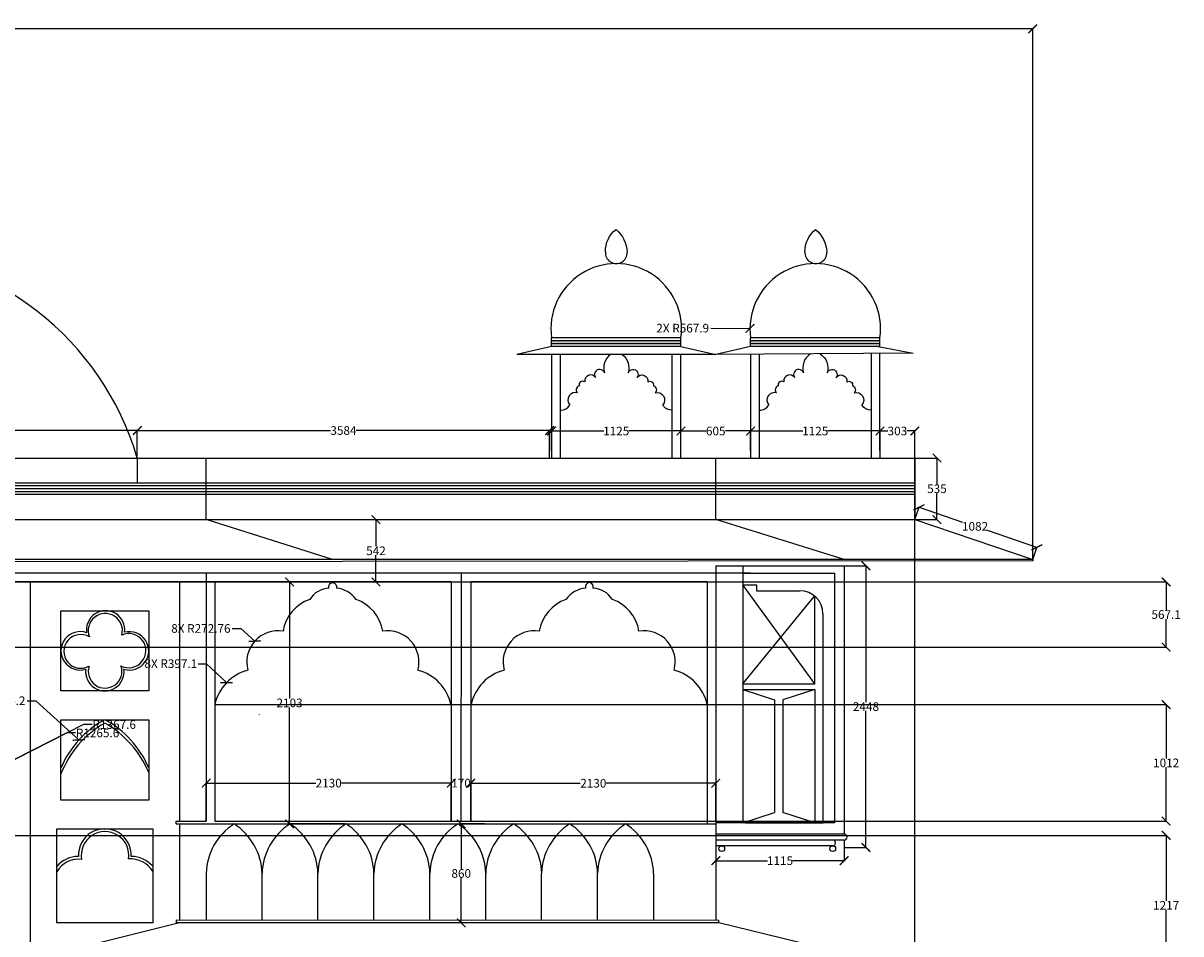
# Model space of a CAD drawing. Units: inches. Extents: x 829 to 33356404, y 1874 to 16983.
# Tile 9 of 9: x 16199 to 26262, y 9069 to 16983. Entities that reach past the tile are written whole.
import ezdxf

# ---------------------------------------------------------------- set-up
doc = ezdxf.new("R2010")
doc.units = ezdxf.units.IN
doc.header["$MEASUREMENT"] = 0
doc.header["$PDMODE"] = 3
for name, color, linetype, lineweight in [('A-ANNO-DIMS', 2, 'Continuous', 18), ('A-ELEV', 7, 'Continuous', 25), ('A-ELEV-PATT', 8, 'Continuous', 13)]:
    doc.layers.add(name, color=color, linetype=linetype, lineweight=lineweight)
doc.styles.get("Standard").update_dxf_attribs({"font": 'arial.ttf'})
doc.dimstyles.get("Standard").update_dxf_attribs({"dimtxt": 75, "dimasz": 75, "dimexe": 0.18, "dimexo": 0.0625, "dimgap": 0.09, "dimtad": 0, "dimtih": 1, "dimtoh": 1, "dimdec": 0, "dimzin": 0, "dimdsep": 46, "dimtxsty": 'Standard', "dimblk": 'ARCHTICK', "dimcen": 0.09, "dimadec": 0, "dimazin": 0, "dimtfac": 1, "dimtdec": 0, "dimtofl": 0, "dimtmove": 0, "dimatfit": 3, "dimfxl": 1, "dimtolj": 1, "dimtzin": 0, "dimarcsym": 0})

# ---------------------------------------------------------------- blocks, each defined once
blk = doc.blocks.new('_ArchTick')
at = {"color": 0, "linetype": 'ByBlock', "const_width": 0.15}
blk.add_lwpolyline([(-0.5, -0.5), (0.5, 0.5)], dxfattribs=at)
blk = doc.blocks.new('*D14')
at = {"layer": 'A-ANNO-DIMS', "color": 0, "lineweight": -2, "transparency": 16777216}
for p, q in [((18994, 12127), (18515, 12127)), ((18515, 12127), (18515, 11114)), ((18515, 10024), (18515, 11037)), ((18994, 10024), (18515, 10024))]:
    blk.add_line(p, q, dxfattribs=at)
at = {"layer": 'Defpoints', "color": 0, "transparency": 16777216}
for p in [(18515, 12127), (18994, 12127), (18994, 10024)]:
    blk.add_point(p, dxfattribs=at)
at = {"layer": 'A-ANNO-DIMS', "color": 0, "lineweight": -2, "transparency": 16777216, "xscale": 75, "yscale": 75, "zscale": 75}
for p, rotation in [((18515, 12127), 90), ((18515, 10024), 270)]:
    blk.add_blockref('_ArchTick', p, dxfattribs=dict(at, rotation=rotation))
at = {"layer": 'A-ANNO-DIMS', "color": 0, "transparency": 16777216, "insert": (18515, 11076), "char_height": 75, "attachment_point": 5}
blk.add_mtext('\\A1;2103', dxfattribs=at)
blk = doc.blocks.new('*D15')
at = {"layer": 'A-ANNO-DIMS', "color": 0, "lineweight": -2, "transparency": 16777216}
for p, q in [((23335, 9884), (23335, 9705)), ((22220, 9819), (22220, 9705)), ((22220, 9705), (22669, 9705)), ((23335, 9705), (22887, 9705))]:
    blk.add_line(p, q, dxfattribs=at)
at = {"layer": 'Defpoints', "color": 0, "transparency": 16777216}
for p in [(23335, 9884), (22220, 9820), (23335, 9705)]:
    blk.add_point(p, dxfattribs=at)
at = {"layer": 'A-ANNO-DIMS', "color": 0, "lineweight": -2, "transparency": 16777216, "xscale": 75, "yscale": 75, "zscale": 75, "rotation": 180}
blk.add_blockref('_ArchTick', (22220, 9705), dxfattribs=at)
at = {"layer": 'A-ANNO-DIMS', "color": 0, "lineweight": -2, "transparency": 16777216, "xscale": 75, "yscale": 75, "zscale": 75}
blk.add_blockref('_ArchTick', (23335, 9705), dxfattribs=at)
at = {"layer": 'A-ANNO-DIMS', "color": 0, "transparency": 16777216, "insert": (22778, 9705), "char_height": 75, "attachment_point": 5}
blk.add_mtext('\\A1;1115', dxfattribs=at)
blk = doc.blocks.new('*D16')
at = {"layer": 'A-ANNO-DIMS', "color": 0, "lineweight": -2, "transparency": 16777216}
for p, q in [((23336, 12268), (23526, 12268)), ((23525, 12268), (23525, 11082)), ((23525, 9820), (23525, 11006)), ((23336, 9820), (23526, 9820))]:
    blk.add_line(p, q, dxfattribs=at)
at = {"layer": 'Defpoints', "color": 0, "transparency": 16777216}
for p in [(23335, 12268), (23525, 12268), (23335, 9820)]:
    blk.add_point(p, dxfattribs=at)
at = {"layer": 'A-ANNO-DIMS', "color": 0, "lineweight": -2, "transparency": 16777216, "xscale": 75, "yscale": 75, "zscale": 75}
for p, rotation in [((23525, 12268), 90), ((23525, 9820), 270)]:
    blk.add_blockref('_ArchTick', p, dxfattribs=dict(at, rotation=rotation))
at = {"layer": 'A-ANNO-DIMS', "color": 0, "transparency": 16777216, "insert": (23525, 11044), "char_height": 75, "attachment_point": 5}
blk.add_mtext('\\A1;2448', dxfattribs=at)
blk = doc.blocks.new('*D25')
at = {"layer": 'A-ANNO-DIMS', "color": 0, "lineweight": -2, "transparency": 16777216}
for p, q in [((20090, 10049), (20090, 10379)), ((20090, 10378), (21042, 10378)), ((22220, 10378), (21268, 10378)), ((22220, 10049), (22220, 10379))]:
    blk.add_line(p, q, dxfattribs=at)
at = {"layer": 'Defpoints', "color": 0, "transparency": 16777216}
for p in [(22220, 10378), (20090, 10049), (22220, 10049)]:
    blk.add_point(p, dxfattribs=at)
at = {"layer": 'A-ANNO-DIMS', "color": 0, "lineweight": -2, "transparency": 16777216, "xscale": 75, "yscale": 75, "zscale": 75, "rotation": 180}
blk.add_blockref('_ArchTick', (20090, 10378), dxfattribs=at)
at = {"layer": 'A-ANNO-DIMS', "color": 0, "lineweight": -2, "transparency": 16777216, "xscale": 75, "yscale": 75, "zscale": 75}
blk.add_blockref('_ArchTick', (22220, 10378), dxfattribs=at)
at = {"layer": 'A-ANNO-DIMS', "color": 0, "transparency": 16777216, "insert": (21155, 10378), "char_height": 75, "attachment_point": 5}
blk.add_mtext('\\A1;2130', dxfattribs=at)
blk = doc.blocks.new('*D26')
at = {"layer": 'A-ANNO-DIMS', "color": 0, "lineweight": -2, "transparency": 16777216}
for p, q in [((17790, 10049), (17790, 10379)), ((17790, 10379), (18742, 10379)), ((19920, 10379), (18967, 10379)), ((19920, 10049), (19920, 10379))]:
    blk.add_line(p, q, dxfattribs=at)
at = {"layer": 'Defpoints', "color": 0, "transparency": 16777216}
for p in [(19920, 10379), (17790, 10049), (19920, 10049)]:
    blk.add_point(p, dxfattribs=at)
at = {"layer": 'A-ANNO-DIMS', "color": 0, "lineweight": -2, "transparency": 16777216, "xscale": 75, "yscale": 75, "zscale": 75, "rotation": 180}
blk.add_blockref('_ArchTick', (17790, 10379), dxfattribs=at)
at = {"layer": 'A-ANNO-DIMS', "color": 0, "lineweight": -2, "transparency": 16777216, "xscale": 75, "yscale": 75, "zscale": 75}
blk.add_blockref('_ArchTick', (19920, 10379), dxfattribs=at)
at = {"layer": 'A-ANNO-DIMS', "color": 0, "transparency": 16777216, "insert": (18855, 10379), "char_height": 75, "attachment_point": 5}
blk.add_mtext('\\A1;2130', dxfattribs=at)
blk = doc.blocks.new('*D27')
at = {"layer": 'A-ANNO-DIMS', "color": 0, "lineweight": -2, "transparency": 16777216}
for p, q in [((19920, 10049), (19920, 10379)), ((19920, 10379), (19926, 10379)), ((20090, 10379), (20084, 10379)), ((20090, 10049), (20090, 10379))]:
    blk.add_line(p, q, dxfattribs=at)
at = {"layer": 'Defpoints', "color": 0, "transparency": 16777216}
for p in [(20090, 10379), (19920, 10049), (20090, 10049)]:
    blk.add_point(p, dxfattribs=at)
at = {"layer": 'A-ANNO-DIMS', "color": 0, "lineweight": -2, "transparency": 16777216, "xscale": 75, "yscale": 75, "zscale": 75, "rotation": 180}
blk.add_blockref('_ArchTick', (19920, 10379), dxfattribs=at)
at = {"layer": 'A-ANNO-DIMS', "color": 0, "lineweight": -2, "transparency": 16777216, "xscale": 75, "yscale": 75, "zscale": 75}
blk.add_blockref('_ArchTick', (20090, 10379), dxfattribs=at)
at = {"layer": 'A-ANNO-DIMS', "color": 0, "transparency": 16777216, "insert": (20005, 10379), "char_height": 75, "attachment_point": 5}
blk.add_mtext('\\A1;170', dxfattribs=at)
blk = doc.blocks.new('*D28')
at = {"layer": 'A-ANNO-DIMS', "color": 0, "lineweight": -2, "transparency": 16777216}
for p, q in [((19162, 12669), (19266, 12669)), ((19266, 12669), (19266, 12437)), ((19266, 12127), (19266, 12360)), ((19162, 12127), (19266, 12127))]:
    blk.add_line(p, q, dxfattribs=at)
at = {"layer": 'Defpoints', "color": 0, "transparency": 16777216}
for p in [(19162, 12669), (19266, 12669), (19162, 12127)]:
    blk.add_point(p, dxfattribs=at)
at = {"layer": 'A-ANNO-DIMS', "color": 0, "lineweight": -2, "transparency": 16777216, "xscale": 75, "yscale": 75, "zscale": 75}
for p, rotation in [((19266, 12669), 90), ((19266, 12127), 270)]:
    blk.add_blockref('_ArchTick', p, dxfattribs=dict(at, rotation=rotation))
at = {"layer": 'A-ANNO-DIMS', "color": 0, "transparency": 16777216, "insert": (19266, 12398), "char_height": 75, "attachment_point": 5}
blk.add_mtext('\\A1;542', dxfattribs=at)
blk = doc.blocks.new('*D50')
at = {"layer": 'A-ANNO-DIMS', "color": 0, "lineweight": -2, "transparency": 16777216}
for p, q in [((22522, 13270), (22522, 13439)), ((22522, 13439), (22975, 13439)), ((23647, 13439), (23193, 13439)), ((23647, 13270), (23647, 13439))]:
    blk.add_line(p, q, dxfattribs=at)
at = {"layer": 'Defpoints', "color": 0, "transparency": 16777216}
for p in [(22522, 13439), (22522, 13269), (23647, 13269)]:
    blk.add_point(p, dxfattribs=at)
at = {"layer": 'A-ANNO-DIMS', "color": 0, "lineweight": -2, "transparency": 16777216, "xscale": 75, "yscale": 75, "zscale": 75, "rotation": 180}
blk.add_blockref('_ArchTick', (22522, 13439), dxfattribs=at)
at = {"layer": 'A-ANNO-DIMS', "color": 0, "lineweight": -2, "transparency": 16777216, "xscale": 75, "yscale": 75, "zscale": 75}
blk.add_blockref('_ArchTick', (23647, 13439), dxfattribs=at)
at = {"layer": 'A-ANNO-DIMS', "color": 0, "transparency": 16777216, "insert": (23084, 13439), "char_height": 75, "attachment_point": 5}
blk.add_mtext('\\A1;1125', dxfattribs=at)
blk = doc.blocks.new('*D49')
at = {"layer": 'A-ANNO-DIMS', "color": 0, "lineweight": -2, "transparency": 16777216}
for p, q in [((21917, 13270), (21917, 13439)), ((21917, 13439), (22136, 13439)), ((22522, 13439), (22303, 13439)), ((22522, 13270), (22522, 13439))]:
    blk.add_line(p, q, dxfattribs=at)
at = {"layer": 'Defpoints', "color": 0, "transparency": 16777216}
for p in [(21917, 13439), (21917, 13269), (22522, 13269)]:
    blk.add_point(p, dxfattribs=at)
at = {"layer": 'A-ANNO-DIMS', "color": 0, "lineweight": -2, "transparency": 16777216, "xscale": 75, "yscale": 75, "zscale": 75, "rotation": 180}
blk.add_blockref('_ArchTick', (21917, 13439), dxfattribs=at)
at = {"layer": 'A-ANNO-DIMS', "color": 0, "lineweight": -2, "transparency": 16777216, "xscale": 75, "yscale": 75, "zscale": 75}
blk.add_blockref('_ArchTick', (22522, 13439), dxfattribs=at)
at = {"layer": 'A-ANNO-DIMS', "color": 0, "transparency": 16777216, "insert": (22219, 13439), "char_height": 75, "attachment_point": 5}
blk.add_mtext('\\A1;605', dxfattribs=at)
blk = doc.blocks.new('*D51')
at = {"layer": 'A-ANNO-DIMS', "color": 0, "lineweight": -2, "transparency": 16777216}
for p, q in [((20792, 13270), (20792, 13439)), ((20792, 13439), (21245, 13439)), ((21917, 13439), (21463, 13439)), ((21917, 13270), (21917, 13439))]:
    blk.add_line(p, q, dxfattribs=at)
at = {"layer": 'Defpoints', "color": 0, "transparency": 16777216}
for p in [(20792, 13439), (20792, 13269), (21917, 13269)]:
    blk.add_point(p, dxfattribs=at)
at = {"layer": 'A-ANNO-DIMS', "color": 0, "lineweight": -2, "transparency": 16777216, "xscale": 75, "yscale": 75, "zscale": 75, "rotation": 180}
blk.add_blockref('_ArchTick', (20792, 13439), dxfattribs=at)
at = {"layer": 'A-ANNO-DIMS', "color": 0, "lineweight": -2, "transparency": 16777216, "xscale": 75, "yscale": 75, "zscale": 75}
blk.add_blockref('_ArchTick', (21917, 13439), dxfattribs=at)
at = {"layer": 'A-ANNO-DIMS', "color": 0, "transparency": 16777216, "insert": (21354, 13439), "char_height": 75, "attachment_point": 5}
blk.add_mtext('\\A1;1125', dxfattribs=at)
blk = doc.blocks.new('*D52')
at = {"layer": 'A-ANNO-DIMS', "color": 0, "lineweight": -2, "transparency": 16777216}
for p, q in [((23950, 12669), (23986, 12776)), ((23986, 12776), (24365, 12647)), ((25010, 12428), (24581, 12574)), ((24974, 12321), (25010, 12428))]:
    blk.add_line(p, q, dxfattribs=at)
at = {"layer": 'Defpoints', "color": 0, "transparency": 16777216}
for p in [(23950, 12669), (25010, 12428), (24974, 12321)]:
    blk.add_point(p, dxfattribs=at)
at = {"layer": 'A-ANNO-DIMS', "color": 0, "lineweight": -2, "transparency": 16777216, "xscale": 75, "yscale": 75, "zscale": 75}
for p, rotation in [((23986, 12776), 161.2250279708252), ((25010, 12428), 341.2250279708252)]:
    blk.add_blockref('_ArchTick', p, dxfattribs=dict(at, rotation=rotation))
at = {"layer": 'A-ANNO-DIMS', "color": 0, "transparency": 16777216, "insert": (24473, 12610), "char_height": 75, "attachment_point": 5}
blk.add_mtext('\\A1;1082', dxfattribs=at)
blk = doc.blocks.new('*D53')
at = {"layer": 'A-ANNO-DIMS', "color": 0, "lineweight": -2, "transparency": 16777216}
for p, q in [((23950, 13204), (24142, 13204)), ((24142, 13204), (24142, 12975)), ((24142, 12669), (24142, 12898)), ((23950, 12669), (24142, 12669))]:
    blk.add_line(p, q, dxfattribs=at)
at = {"layer": 'Defpoints', "color": 0, "transparency": 16777216}
for p in [(23950, 13204), (23950, 12669), (24142, 12669)]:
    blk.add_point(p, dxfattribs=at)
at = {"layer": 'A-ANNO-DIMS', "color": 0, "lineweight": -2, "transparency": 16777216, "xscale": 75, "yscale": 75, "zscale": 75}
for p, rotation in [((24142, 13204), 90), ((24142, 12669), 270)]:
    blk.add_blockref('_ArchTick', p, dxfattribs=dict(at, rotation=rotation))
at = {"layer": 'A-ANNO-DIMS', "color": 0, "transparency": 16777216, "insert": (24142, 12937), "char_height": 75, "attachment_point": 5}
blk.add_mtext('\\A1;535', dxfattribs=at)
blk = doc.blocks.new('*D55')
at = {"layer": 'A-ANNO-DIMS', "color": 0, "lineweight": -2, "transparency": 16777216}
for p, q in [((9931, 13204), (9931, 13443)), ((9931, 13443), (13449, 13443)), ((17191, 13443), (13672, 13443)), ((17191, 13204), (17191, 13443))]:
    blk.add_line(p, q, dxfattribs=at)
at = {"layer": 'Defpoints', "color": 0, "transparency": 16777216}
for p in [(17191, 13443), (9931, 13204), (17191, 13204)]:
    blk.add_point(p, dxfattribs=at)
at = {"layer": 'A-ANNO-DIMS', "color": 0, "lineweight": -2, "transparency": 16777216, "xscale": 75, "yscale": 75, "zscale": 75, "rotation": 180}
blk.add_blockref('_ArchTick', (9931, 13443), dxfattribs=at)
at = {"layer": 'A-ANNO-DIMS', "color": 0, "lineweight": -2, "transparency": 16777216, "xscale": 75, "yscale": 75, "zscale": 75}
blk.add_blockref('_ArchTick', (17191, 13443), dxfattribs=at)
at = {"layer": 'A-ANNO-DIMS', "color": 0, "transparency": 16777216, "insert": (13561, 13443), "char_height": 75, "attachment_point": 5}
blk.add_mtext('\\A1;7260', dxfattribs=at)
blk = doc.blocks.new('*D58')
at = {"layer": 'A-ANNO-DIMS', "color": 0, "lineweight": -2, "transparency": 16777216}
for p, q in [((23647, 13204), (23647, 13439)), ((23647, 13439), (23715, 13439)), ((23950, 13439), (23881, 13439)), ((23950, 13204), (23950, 13439))]:
    blk.add_line(p, q, dxfattribs=at)
at = {"layer": 'Defpoints', "color": 0, "transparency": 16777216}
for p in [(23647, 13439), (23647, 13204), (23950, 13204)]:
    blk.add_point(p, dxfattribs=at)
at = {"layer": 'A-ANNO-DIMS', "color": 0, "lineweight": -2, "transparency": 16777216, "xscale": 75, "yscale": 75, "zscale": 75, "rotation": 180}
blk.add_blockref('_ArchTick', (23647, 13439), dxfattribs=at)
at = {"layer": 'A-ANNO-DIMS', "color": 0, "lineweight": -2, "transparency": 16777216, "xscale": 75, "yscale": 75, "zscale": 75}
blk.add_blockref('_ArchTick', (23950, 13439), dxfattribs=at)
at = {"layer": 'A-ANNO-DIMS', "color": 0, "transparency": 16777216, "insert": (23798, 13439), "char_height": 75, "attachment_point": 5}
blk.add_mtext('\\A1;303', dxfattribs=at)
blk = doc.blocks.new('*D65')
at = {"layer": 'A-ANNO-DIMS', "color": 0, "lineweight": -2, "transparency": 16777216}
for p, q in [((20209, 10024), (20007, 10024)), ((20007, 10024), (20007, 9632)), ((20007, 9164), (20007, 9556)), ((20209, 9164), (20007, 9164))]:
    blk.add_line(p, q, dxfattribs=at)
at = {"layer": 'Defpoints', "color": 0, "transparency": 16777216}
for p in [(20209, 10024), (20007, 9164), (20209, 9164)]:
    blk.add_point(p, dxfattribs=at)
at = {"layer": 'A-ANNO-DIMS', "color": 0, "lineweight": -2, "transparency": 16777216, "xscale": 75, "yscale": 75, "zscale": 75}
for p, rotation in [((20007, 10024), 90), ((20007, 9164), 270)]:
    blk.add_blockref('_ArchTick', p, dxfattribs=dict(at, rotation=rotation))
at = {"layer": 'A-ANNO-DIMS', "color": 0, "transparency": 16777216, "insert": (20007, 9594), "char_height": 75, "attachment_point": 5}
blk.add_mtext('\\A1;860', dxfattribs=at)
blk = doc.blocks.new('*D66')
at = {"layer": 'A-ANNO-DIMS', "color": 0, "lineweight": -2, "transparency": 16777216}
for p, q in [((17191, 13204), (17191, 13443)), ((17191, 13443), (18871, 13443)), ((20775, 13443), (19095, 13443)), ((20775, 13204), (20775, 13443))]:
    blk.add_line(p, q, dxfattribs=at)
at = {"layer": 'Defpoints', "color": 0, "transparency": 16777216}
for p in [(20775, 13443), (17191, 13204), (20775, 13204)]:
    blk.add_point(p, dxfattribs=at)
at = {"layer": 'A-ANNO-DIMS', "color": 0, "lineweight": -2, "transparency": 16777216, "xscale": 75, "yscale": 75, "zscale": 75, "rotation": 180}
blk.add_blockref('_ArchTick', (17191, 13443), dxfattribs=at)
at = {"layer": 'A-ANNO-DIMS', "color": 0, "lineweight": -2, "transparency": 16777216, "xscale": 75, "yscale": 75, "zscale": 75}
blk.add_blockref('_ArchTick', (20775, 13443), dxfattribs=at)
at = {"layer": 'A-ANNO-DIMS', "color": 0, "transparency": 16777216, "insert": (18983, 13443), "char_height": 75, "attachment_point": 5}
blk.add_mtext('\\A1;3584', dxfattribs=at)
blk = doc.blocks.new('ARCADE-ARCHES')
for p, q in [((0, 405), (0, 0)), ((486, 0), (486, 405)), ((972, 0), (972, 405)), ((1458, 0), (1458, 405)), ((1944, 0), (1944, 405)), ((2430, 0), (2430, 405)), ((2916, 0), (2916, 405)), ((3402, 0), (3402, 405)), ((3889, 405), (3889, 0))]:
    blk.add_line(p, q)
for centre, start, end in [((526, 392), 122.5147, 178.5225), ((-40, 392), 1.4775, 57.4853), ((1012, 392), 122.5147, 178.5225), ((446, 392), 1.4775, 57.4853), ((1498, 392), 122.5147, 178.5225), ((933, 392), 1.4775, 57.4853), ((1984, 392), 122.5147, 178.5225), ((1419, 392), 1.4775, 57.4853), ((2470, 392), 122.5147, 178.5225), ((1905, 392), 1.4775, 57.4853), ((2956, 392), 122.5147, 178.5225), ((2391, 392), 1.4775, 57.4853), ((3442, 392), 122.5147, 178.5225), ((2877, 392), 1.4775, 57.4853), ((3928, 392), 122.5147, 178.5225), ((3363, 392), 1.4775, 57.4853)]:
    blk.add_arc(centre, 526, start, end)
blk = doc.blocks.new('CHHATRI-ARCH-A')
blk.add_lwpolyline([(0, 0, 0.306755), (82, 44, 10.100933)], format="xyb")
for centre, radius, start, end in [((525, 365), 147, 122.4143, 196.9076), ((264, 253), 51.8, 32.9883, 190.2779), ((342, 309), 44.1, 17.6268, 218.3613), ((175, 175), 36.4, 106.3078, 227.8776), ((195, 218), 31.7, 54.8887, 193.7899), ((131, 87), 64.5, 72.3169, 221.8651)]:
    blk.add_arc(centre, radius, start, end)
blk = doc.blocks.new('CHHATRI-ARCH-B')
blk.add_lwpolyline([(0, 0, 0.306755), (82, 44, 10.100933)], format="xyb")
for centre, radius, start, end in [((525, 365), 147, 126.8528, 196.9076), ((264, 253), 51.8, 32.9883, 190.2779), ((342, 309), 44.1, 17.6268, 218.3613), ((175, 175), 36.4, 106.3078, 227.8776), ((195, 218), 31.7, 54.8887, 193.7899), ((131, 87), 64.5, 72.3169, 221.8651)]:
    blk.add_arc(centre, radius, start, end)
blk = doc.blocks.new('*D82')
at = {"layer": 'A-ANNO-DIMS', "color": 0, "lineweight": -2, "transparency": 16777216}
for p, q in [((2146, 12292), (2146, 16934)), ((2146, 16934), (13418, 16934)), ((24974, 16934), (13702, 16934)), ((24974, 12321), (24974, 16934))]:
    blk.add_line(p, q, dxfattribs=at)
at = {"layer": 'Defpoints', "color": 0, "transparency": 16777216}
for p in [(24974, 16934), (2146, 12292), (24974, 12321)]:
    blk.add_point(p, dxfattribs=at)
at = {"layer": 'A-ANNO-DIMS', "color": 0, "lineweight": -2, "transparency": 16777216, "xscale": 75, "yscale": 75, "zscale": 75, "rotation": 180}
blk.add_blockref('_ArchTick', (2146, 16934), dxfattribs=at)
at = {"layer": 'A-ANNO-DIMS', "color": 0, "lineweight": -2, "transparency": 16777216, "xscale": 75, "yscale": 75, "zscale": 75}
blk.add_blockref('_ArchTick', (24974, 16934), dxfattribs=at)
at = {"layer": 'A-ANNO-DIMS', "color": 0, "transparency": 16777216, "insert": (13560, 16934), "char_height": 75, "attachment_point": 5}
blk.add_mtext('\\A1;22828', dxfattribs=at)
blk = doc.blocks.new('*D90')
at = {"layer": 'A-ANNO-DIMS', "color": 0, "lineweight": -2, "transparency": 16777216}
for p, q in [((17865, 11061), (26134, 11061)), ((26134, 11061), (26134, 10594)), ((26134, 10049), (26134, 10517)), ((17865, 10049), (26134, 10049))]:
    blk.add_line(p, q, dxfattribs=at)
at = {"layer": 'Defpoints', "color": 0, "transparency": 16777216}
for p in [(17865, 11061), (26134, 11061), (17865, 10049)]:
    blk.add_point(p, dxfattribs=at)
at = {"layer": 'A-ANNO-DIMS', "color": 0, "lineweight": -2, "transparency": 16777216, "xscale": 75, "yscale": 75, "zscale": 75}
for p, rotation in [((26134, 11061), 90), ((26134, 10049), 270)]:
    blk.add_blockref('_ArchTick', p, dxfattribs=dict(at, rotation=rotation))
at = {"layer": 'A-ANNO-DIMS', "color": 0, "transparency": 16777216, "insert": (26134, 10555), "char_height": 75, "attachment_point": 5}
blk.add_mtext('\\A1;1012', dxfattribs=at)
blk = doc.blocks.new('*D91')
at = {"layer": 'A-ANNO-DIMS', "color": 0, "lineweight": -2, "transparency": 16777216}
for p, q in [((11082, 9925), (26134, 9925)), ((26134, 9925), (26134, 9355)), ((26134, 8708), (26134, 9279)), ((11082, 8708), (26134, 8708))]:
    blk.add_line(p, q, dxfattribs=at)
at = {"layer": 'Defpoints', "color": 0, "transparency": 16777216}
for p in [(11082, 9925), (11082, 8708), (26134, 8708)]:
    blk.add_point(p, dxfattribs=at)
at = {"layer": 'A-ANNO-DIMS', "color": 0, "lineweight": -2, "transparency": 16777216, "xscale": 75, "yscale": 75, "zscale": 75}
for p, rotation in [((26134, 9925), 90), ((26134, 8708), 270)]:
    blk.add_blockref('_ArchTick', p, dxfattribs=dict(at, rotation=rotation))
at = {"layer": 'A-ANNO-DIMS', "color": 0, "transparency": 16777216, "insert": (26134, 9317), "char_height": 75, "attachment_point": 5}
blk.add_mtext('\\A1;1217', dxfattribs=at)
blk = doc.blocks.new('*D93')
at = {"layer": 'A-ANNO-DIMS', "color": 0, "lineweight": -2, "transparency": 16777216}
for p, q in [((10980, 12127), (26134, 12127)), ((26134, 12127), (26134, 11882)), ((26134, 11560), (26134, 11805)), ((11677, 11560), (26134, 11560))]:
    blk.add_line(p, q, dxfattribs=at)
at = {"layer": 'Defpoints', "color": 0, "transparency": 16777216}
for p in [(10980, 12127), (11677, 11560), (26134, 11560)]:
    blk.add_point(p, dxfattribs=at)
at = {"layer": 'A-ANNO-DIMS', "color": 0, "lineweight": -2, "transparency": 16777216, "xscale": 75, "yscale": 75, "zscale": 75}
for p, rotation in [((26134, 12127), 90), ((26134, 11560), 270)]:
    blk.add_blockref('_ArchTick', p, dxfattribs=dict(at, rotation=rotation))
at = {"layer": 'A-ANNO-DIMS', "color": 0, "transparency": 16777216, "insert": (26134, 11844), "char_height": 75, "attachment_point": 5}
blk.add_mtext('\\A1;567.1', dxfattribs=at)
blk = doc.blocks.new('*D110')
at = {"layer": 'A-ANNO-DIMS', "color": 0, "lineweight": -2, "transparency": 16777216}
for p, q in [((17719, 11417), (17794, 11417)), ((17794, 11417), (17966, 11252)), ((18253, 10977), (18253, 10977)), ((18253, 10976), (18253, 10977))]:
    blk.add_line(p, q, dxfattribs=at)
at = {"layer": 'Defpoints', "color": 0, "transparency": 16777216}
for p in [(17966, 11252), (18253, 10977)]:
    blk.add_point(p, dxfattribs=at)
at = {"layer": 'A-ANNO-DIMS', "color": 0, "lineweight": -2, "transparency": 16777216, "xscale": 75, "yscale": 75, "zscale": 75, "rotation": 316.167768460209}
blk.add_blockref('_ArchTick', (17966, 11252), dxfattribs=at)
at = {"layer": 'A-ANNO-DIMS', "color": 0, "transparency": 16777216, "insert": (17483, 11417), "char_height": 75, "attachment_point": 5}
blk.add_mtext('\\A1;8X R397.1', dxfattribs=at)
blk = doc.blocks.new('*D112')
at = {"layer": 'A-ANNO-DIMS', "color": 0, "lineweight": -2, "transparency": 16777216}
for p, q in [((18017, 11723), (18092, 11723)), ((18092, 11723), (18213, 11613)), ((18416, 11431), (18416, 11431)), ((18416, 11431), (18416, 11431))]:
    blk.add_line(p, q, dxfattribs=at)
at = {"layer": 'Defpoints', "color": 0, "transparency": 16777216}
for p in [(18213, 11613), (18416, 11431)]:
    blk.add_point(p, dxfattribs=at)
at = {"layer": 'A-ANNO-DIMS', "color": 0, "lineweight": -2, "transparency": 16777216, "xscale": 75, "yscale": 75, "zscale": 75, "rotation": 317.9756692368}
blk.add_blockref('_ArchTick', (18213, 11613), dxfattribs=at)
at = {"layer": 'A-ANNO-DIMS', "color": 0, "transparency": 16777216, "insert": (17744, 11723), "char_height": 75, "attachment_point": 5}
blk.add_mtext('\\A1;8X R272.76', dxfattribs=at)
blk = doc.blocks.new('*D115')
at = {"layer": 'A-ANNO-DIMS', "color": 0, "lineweight": -2, "transparency": 16777216}
for p, q in [((22176, 14333), (22516, 14330)), ((23084, 14326), (23084, 14326)), ((23084, 14326), (23084, 14326))]:
    blk.add_line(p, q, dxfattribs=at)
at = {"layer": 'Defpoints', "color": 0, "transparency": 16777216}
for p in [(22516, 14330), (23084, 14326)]:
    blk.add_point(p, dxfattribs=at)
at = {"layer": 'A-ANNO-DIMS', "color": 0, "lineweight": -2, "transparency": 16777216, "xscale": 75, "yscale": 75, "zscale": 75, "rotation": 359.558569188689}
blk.add_blockref('_ArchTick', (22516, 14330), dxfattribs=at)
at = {"layer": 'A-ANNO-DIMS', "color": 0, "transparency": 16777216, "insert": (21932, 14333), "char_height": 75, "attachment_point": 5}
blk.add_mtext('\\A1;2X R567.9', dxfattribs=at)
blk = doc.blocks.new('*D125')
at = {"layer": 'A-ANNO-DIMS', "color": 0, "lineweight": -2, "transparency": 16777216}
for p, q in [((16725, 10888), (15993, 10518)), ((16800, 10888), (16725, 10888)), ((14772, 9900), (14773, 9900)), ((14772, 9900), (14772, 9900))]:
    blk.add_line(p, q, dxfattribs=at)
at = {"layer": 'Defpoints', "color": 0, "transparency": 16777216}
for p in [(15993, 10518), (14772, 9900)]:
    blk.add_point(p, dxfattribs=at)
at = {"layer": 'A-ANNO-DIMS', "color": 0, "lineweight": -2, "transparency": 16777216, "xscale": 75, "yscale": 75, "zscale": 75, "rotation": 206.8466405163161}
blk.add_blockref('_ArchTick', (15993, 10518), dxfattribs=at)
at = {"layer": 'A-ANNO-DIMS', "color": 0, "transparency": 16777216, "insert": (16991, 10888), "char_height": 75, "attachment_point": 5}
blk.add_mtext('\\A1;R1367.6', dxfattribs=at)
blk = doc.blocks.new('*D126')
at = {"layer": 'A-ANNO-DIMS', "color": 0, "lineweight": -2, "transparency": 16777216}
for p, q in [((16579, 10815), (15902, 10472)), ((16654, 10815), (16579, 10815)), ((14772, 9900), (14773, 9900)), ((14772, 9900), (14772, 9900))]:
    blk.add_line(p, q, dxfattribs=at)
at = {"layer": 'Defpoints', "color": 0, "transparency": 16777216}
for p in [(15902, 10472), (14772, 9900)]:
    blk.add_point(p, dxfattribs=at)
at = {"layer": 'A-ANNO-DIMS', "color": 0, "lineweight": -2, "transparency": 16777216, "xscale": 75, "yscale": 75, "zscale": 75, "rotation": 206.8466187545911}
blk.add_blockref('_ArchTick', (15902, 10472), dxfattribs=at)
at = {"layer": 'A-ANNO-DIMS', "color": 0, "transparency": 16777216, "insert": (16846, 10815), "char_height": 75, "attachment_point": 5}
blk.add_mtext('\\A1;R1265.6', dxfattribs=at)
blk = doc.blocks.new('*D130')
at = {"layer": 'A-ANNO-DIMS', "color": 0, "lineweight": -2, "transparency": 16777216}
for p, q in [((16233, 11095), (16308, 11095)), ((16308, 11095), (16683, 10754)), ((17306, 10185), (17306, 10185)), ((17306, 10185), (17306, 10185))]:
    blk.add_line(p, q, dxfattribs=at)
at = {"layer": 'Defpoints', "color": 0, "transparency": 16777216}
for p in [(16683, 10754), (17306, 10185)]:
    blk.add_point(p, dxfattribs=at)
at = {"layer": 'A-ANNO-DIMS', "color": 0, "lineweight": -2, "transparency": 16777216, "xscale": 75, "yscale": 75, "zscale": 75, "rotation": 317.6357309782866}
blk.add_blockref('_ArchTick', (16683, 10754), dxfattribs=at)
at = {"layer": 'A-ANNO-DIMS', "color": 0, "transparency": 16777216, "insert": (15989, 11095), "char_height": 75, "attachment_point": 5}
blk.add_mtext('\\A1;4X R844.2', dxfattribs=at)

msp = doc.modelspace()

# ---------------------------------------------------------------- hatches: boundary and pattern name
at = {"layer": 'A-ELEV-PATT'}
h = msp.add_hatch(color=256, dxfattribs=at)
h.dxf.hatch_style = 1
h.paths.add_polyline_path([(20791.778, 14222.485), (21354.278, 14222.485), (21354.278, 14197.485), (20791.778, 14197.485)])
h = msp.add_hatch(color=256, dxfattribs=at)
h.dxf.hatch_style = 1
h.paths.add_polyline_path([(21354.278, 14222.485), (21916.778, 14222.485), (21916.778, 14197.485), (21354.278, 14197.485)])
h = msp.add_hatch(color=256, dxfattribs=at)
h.dxf.hatch_style = 1
h.paths.add_polyline_path([(22521.778, 14222.485), (23084.278, 14222.485), (23084.278, 14197.485), (22521.778, 14197.485)])
h = msp.add_hatch(color=256, dxfattribs=at)
h.dxf.hatch_style = 1
h.paths.add_polyline_path([(23084.278, 14222.485), (23646.778, 14222.485), (23646.778, 14197.485), (23084.278, 14197.485)])

# ---------------------------------------------------------------- linework, layer by layer
at = {"layer": 'A-ELEV'}
for p, q in [((21916.778, 14247.485), (20791.778, 14247.485)), ((20791.778, 14172.485), (20791.778, 14247.485)), ((21916.778, 14222.485), (20791.778, 14222.485)), ((21916.778, 14197.485), (20791.778, 14197.485)), ((21916.778, 14172.485), (21916.778, 14247.485)), ((23646.778, 14247.485), (22521.778, 14247.485)), ((22521.778, 14172.485), (22521.778, 14247.485)), ((23646.778, 14222.485), (22521.778, 14222.485)), ((23646.778, 14197.485), (22521.778, 14197.485)), ((23646.778, 14172.485), (23646.778, 14247.485)), ((20791.778, 14172.485), (20489.778, 14103.629)), ((22219.778, 14103.629), (20489.778, 14103.629)), ((21916.778, 14172.485), (20791.778, 14172.485)), ((20791.778, 14103.629), (20791.778, 13204.032)), ((20866.778, 14103.629), (20866.778, 13204.032)), ((21841.778, 13204.032), (21841.778, 14103.629)), ((21916.778, 14172.485), (22219.778, 14103.629)), ((21916.778, 13204.032), (21916.778, 14103.629)), ((23934.855, 14115.977), (22204.855, 14103.629)), ((22521.778, 14172.485), (22219.778, 14103.629)), ((23646.778, 14172.485), (22521.778, 14172.485)), ((22521.778, 14105.785), (22521.778, 13204.032)), ((22596.778, 14106.32), (22596.778, 13204.032)), ((23571.778, 13204.032), (23571.778, 14113.279)), ((23631.855, 14172.485), (23934.855, 14115.977)), ((23646.778, 13269.485), (23646.778, 14113.814)), ((3169.778, 13204.032), (23949.778, 13204.032)), ((17190.778, 13204.032), (17190.778, 12986.532)), ((17789.778, 12669.032), (17789.778, 13204.032)), ((22219.278, 12669.032), (22219.278, 13204.032)), ((23949.778, 4746.468), (23949.778, 13204.032)), ((23949.778, 13204.032), (23949.778, 12669.032)), ((23949.778, 12986.532), (3169.778, 12986.532)), ((23949.778, 12961.532), (3169.778, 12961.532)), ((23949.778, 12936.532), (3169.778, 12936.532)), ((23949.778, 12911.532), (3169.778, 12911.532)), ((23949.778, 12886.532), (3169.778, 12886.532)), ((3169.778, 12669.032), (23949.778, 12669.032)), ((18889.175, 12320.882), (17789.778, 12669.032)), ((23334.312, 12320.882), (22219.278, 12669.032)), ((23949.778, 12669.032), (24973.928, 12320.882)), ((24973.929, 12320.882), (2145.628, 12320.882)), ((24973.929, 12310.744), (2145.651, 12292.214)), ((24973.929, 12320.882), (24973.929, 12310.744)), ((22522.278, 12202.212), (3169.778, 12202.212)), ((17789.778, 12202.212), (17789.778, 10049.392)), ((20005.152, 12202.212), (20004.887, 10049.392)), ((22220.173, 12267.948), (22220.173, 9188.877)), ((22220.173, 12267.948), (23335.46, 12267.948)), ((22453.965, 12267.948), (22453.965, 10034.257)), ((22453.965, 12202.212), (23250.93, 12202.212)), ((23250.93, 12202.212), (23250.93, 10034.257)), ((23335.46, 12267.948), (23335.46, 9934.257)), ((18091.883, 12127.212), (9559.826, 12127.212)), ((16258.701, 12127.212), (16258.701, 5024.468)), ((17559.778, 10049.392), (17559.778, 12127.212)), ((17864.778, 12127.212), (17864.778, 10049.392)), ((19919.89, 12127.212), (17864.778, 12127.212)), ((19919.89, 12127.212), (19919.89, 10049.392)), ((20089.89, 12127.212), (20089.89, 10049.392)), ((22144.778, 12127.212), (20089.89, 12127.212)), ((22144.778, 12127.212), (22144.778, 10023.842)), ((22453.965, 12100.687), (22453.965, 12100.687)), ((22453.965, 12100.687), (22574.779, 12100.687)), ((23079.354, 11242.683), (22453.965, 12100.687)), ((22574.779, 12100.687), (22574.779, 12049.925)), ((22453.965, 11242.683), (23077.598, 12004.701)), ((22574.779, 12049.925), (22574.779, 12049.925)), ((22574.779, 12049.925), (22950.93, 12049.925)), ((23079.331, 11242.683), (23079.331, 12004.367)), ((23150.93, 11849.925), (23150.93, 11754.206)), ((23150.93, 11806.442), (23150.93, 10034.257)), ((22453.965, 11242.683), (23079.354, 11242.683)), ((22453.965, 11242.683), (22453.965, 11242.683)), ((22453.965, 11191.921), (23079.354, 11191.921)), ((22453.965, 11191.921), (22731.126, 11101.847)), ((23079.354, 11191.921), (22802.193, 11101.847)), ((23079.354, 11191.921), (23079.354, 10034.257)), ((22731.126, 11101.847), (22731.126, 10124.33)), ((22802.193, 11101.847), (22802.193, 10124.33)), ((22453.965, 10034.257), (22731.126, 10124.33)), ((23079.354, 10034.257), (22802.193, 10124.33)), ((17530.231, 10049.392), (17789.778, 10049.392)), ((17530.231, 10024.454), (17530.231, 10049.392)), ((17530.231, 10024.454), (22220.173, 10023.833)), ((17559.778, 9189.453), (17559.778, 10024.45)), ((17864.778, 10049.392), (22144.89, 10049.392)), ((23250.93, 10034.257), (22220.46, 10034.257)), ((22476.056, 10034.257), (23152.207, 10034.257)), ((23335.46, 9934.257), (22220.46, 9934.257)), ((23335.46, 9884.257), (22220.46, 9884.257)), ((23235.46, 9834.257), (22220.46, 9834.257)), ((17559.22, 9165.468), (16492.651, 8897.385)), ((17530.231, 9189.457), (22247.133, 9188.874)), ((17530.231, 9189.457), (17530.231, 9165.468)), ((22247.13, 9165.468), (17530.231, 9165.468)), ((22247.13, 9165.468), (22247.133, 9188.874)), ((23335.316, 8897.468), (22247.13, 9165.468))]:
    msp.add_line(p, q, dxfattribs=at)
for points in [[(21259.732, 14996.8, -0.235502326), (21352.151, 15190.287, -0.2104826), (21449.057, 14993.527, -0.234209501)], [(22994.733, 14996.669, -0.235502326), (23087.152, 15190.156, -0.2104826), (23184.058, 14993.397, -0.234209501)], [(21349.279, 14893.654, -0.000002916), (21349.277, 14893.653, -0.000003298), (21349.275, 14893.655)], [(23084.28, 14893.524, -0.000002916), (23084.278, 14893.523, -0.000003298), (23084.276, 14893.524)], [(18856.859, 12073.468, -0.442920108), (18891.241, 12123.624, -0.367737881), (18923.182, 12073.468, -0.247488348)], [(21153.177, 12073.468, 0.442920108), (21118.795, 12123.624, 0.367737881), (21086.854, 12073.468, 0.247488348)]]:
    msp.add_lwpolyline(points, format="xyb", dxfattribs=at)
for points in [[(16528.074, 11877.212), (17290.405, 11877.212), (17290.405, 11179.704), (16528.074, 11179.704)], [(16528.074, 10929.704), (17290.405, 10929.704), (17290.405, 10232.196), (16528.074, 10232.196)], [(16492.651, 9982.196), (17325.828, 9982.196), (17325.828, 9165.468), (16492.651, 9165.468)]]:
    msp.add_lwpolyline(points, close=True, dxfattribs=at)
for centre in [(22271.167, 9809.257), (23235.552, 9809.257)]:
    msp.add_circle(centre, 25, dxfattribs=at)
for centre, radius, start, end in [((14785.821, 12499.606), 2506, 16.3256048, 87.9689122), ((21354.278, 14988.438), 94.915, 174.9458751, 3.0734321), ((23089.279, 14988.308), 94.915, 174.9458751, 3.0734321), ((21354.278, 14325.622), 567.901, 352.0917127, 187.9082873), ((23084.278, 14325.622), 567.901, 352.0917127, 187.9082873), ((18807.214, 11640.647), 354.179, 109.4034394, 170.3116953), ((18866.872, 11865.187), 208.419, 92.0817943, 148.2984828), ((18901.683, 11841.246), 233.215, 34.9091215, 84.7106013), ((18975.269, 11640.647), 354.179, 9.6883047, 70.5965606), ((21034.767, 11640.647), 354.179, 109.4034394, 170.3116953), ((21108.353, 11841.246), 233.215, 95.2893987, 145.0908785), ((21143.164, 11865.187), 208.419, 31.7015172, 87.9182057), ((21202.822, 11640.647), 354.179, 9.6883047, 70.5965606), ((22950.93, 11849.925), 200, 0, 90), ((16915.996, 11710.622), 166.726, 352.8036552, 188.7161935), ((16913.34, 11704.536), 148.406, 344.8754049, 201.7505434), ((16694.801, 11528.458), 166.726, 70.2299001, 287.1891398), ((17117.42, 11530.089), 148.727, 242.8881159, 114.1355922), ((17123.679, 11528.458), 166.726, 252.8108602, 104.6864663), ((18415.703, 11430.806), 272.758, 81.0607154, 194.8907352), ((19366.78, 11430.806), 272.758, 345.1092648, 98.9392846), ((20643.256, 11430.806), 272.758, 81.0607154, 194.8907352), ((21594.333, 11430.806), 272.758, 345.1092648, 98.9392846), ((16699.57, 11523.821), 146.871, 58.8698998, 299.852673), ((16911.373, 11350.379), 146.143, 161.6289467, 18.8945071), ((16909.24, 11346.43), 166.726, 172.1579984, 7.8420016), ((18252.722, 10976.551), 397.12, 104.6768994, 167.65861), ((19529.761, 10976.551), 397.12, 12.34139, 75.3231006), ((20480.275, 10976.551), 397.12, 104.6768994, 167.65861), ((21757.314, 10976.551), 397.12, 12.34139, 75.3231006), ((17306.384, 10184.731), 844.22, 118.0620346, 157.2094631), ((17332.151, 10151.495), 860.805, 119.4258677, 159.0828764), ((16512.095, 10184.731), 844.22, 22.7905369, 61.9379654), ((16457.563, 10115.752), 906.1, 23.1978992, 60.1002346), ((16909.24, 9752.067), 230.168, 357.3160887, 182.6839113), ((16910.573, 9749.866), 207.419, 351.6467456, 189.2312463), ((23235.46, 9859.257), 25, 270, 90), ((23335.46, 9909.257), 25, 270, 90), ((16675.101, 9508.068), 233.259, 88.9625622, 141.4604412), ((16678.821, 9506.158), 212.161, 82.6833719, 151.3414814), ((17132.45, 9492.24), 228.102, 32.0298486, 94.1878817), ((17140.006, 9496.16), 245.131, 40.7070038, 90.1988869)]:
    msp.add_arc(centre, radius, start, end, dxfattribs=at)

# ---------------------------------------------------------------- block references
for name, p in [('CHHATRI-ARCH-B', (20867.778, 13621.512)), ('ARCADE-ARCHES', (17789.673, 9188.901))]:
    msp.add_blockref(name, p, dxfattribs=at)
at = {"layer": 'A-ELEV', "extrusion": (0, 0, -1), "zscale": -1}
for name, p in [('CHHATRI-ARCH-B', (-21841.778, 13621.512)), ('CHHATRI-ARCH-A', (-23571.778, 13621.513))]:
    msp.add_blockref(name, p, dxfattribs=at)
at = {"layer": 'A-ELEV', "rotation": 0.0409553348768901}
msp.add_blockref('CHHATRI-ARCH-A', (22597.845, 13621.386), dxfattribs=at)

# ---------------------------------------------------------------- dimensions: what is measured, and where the dimension line sits
at = {"layer": 'A-ANNO-DIMS'}
for base, p1, p2, override, picture, middle in [((24973.929, 16934.032), (2145.651, 12292.214), (24973.929, 12320.882), {"dimdec": 0, "dimlfac": 1, "dimrnd": 0, "dimzin": 0, "dimdsep": 46, "dimlunit": 2}, '*D82', (13559.79, 16934.032)), ((17190.778, 13442.842), (9930.778, 13204.032), (17190.778, 13204.032), {"dimclrd": 0, "dimclre": 0, "dimclrt": 0}, '*D55', (13560.778, 13442.842)), ((20774.778, 13442.842), (17190.778, 13204.032), (20774.778, 13204.032), {"dimclrd": 0, "dimclre": 0, "dimclrt": 0}, '*D66', (18982.778, 13442.842)), ((23646.778, 13438.732), (23949.778, 13204.032), (23646.778, 13204.032), {"dimclrd": 0, "dimclre": 0, "dimclrt": 0}, '*D58', (23798.278, 13438.732)), ((19919.89, 10378.856), (17789.778, 10049.392), (19919.89, 10049.392), {"dimclrd": 0, "dimclre": 0, "dimclrt": 0}, '*D26', (18854.834, 10378.856)), ((20089.89, 10378.856), (19919.89, 10049.392), (20089.89, 10049.392), {"dimclrd": 0, "dimclre": 0, "dimclrt": 0}, '*D27', (20004.89, 10378.856)), ((22220.173, 10378.476), (20089.89, 10049.392), (22220.173, 10049.392), {"dimclrd": 0, "dimclre": 0, "dimclrt": 0}, '*D25', (21155.031, 10378.476))]:
    dim = msp.add_linear_dim(base=base, p1=p1, p2=p2, dimstyle='Standard', override=override, dxfattribs=at)
    dim.commit()
    dim.dimension.update_dxf_attribs({"geometry": picture, "text_midpoint": middle})
for center, mpoint, text, override, picture, middle in [((23084.278, 14325.622), (22516.394, 14329.997), '2X <>', {"dimdec": 1, "dimlfac": 1, "dimrnd": 0, "dimzin": 0, "dimdsep": 46, "dimlunit": 2}, '*D115', (22175.664, 14332.622)), ((18415.703, 11430.806), (18213.081, 11613.403), '8X <>', {"dimdec": 2, "dimlfac": 1, "dimrnd": 0, "dimzin": 0, "dimdsep": 46, "dimlunit": 2}, '*D112', (17744.249, 11722.961)), ((18252.722, 10976.551), (17966.251, 11251.576), '8X <>', {"dimdec": 1, "dimlfac": 1, "dimrnd": 0, "dimzin": 0, "dimdsep": 46, "dimlunit": 2}, '*D110', (17483.458, 11416.592)), ((17306.384, 10184.731), (16682.61, 10753.602), '4X <>', {"dimdec": 1, "dimlfac": 1, "dimrnd": 0, "dimzin": 0, "dimdsep": 46, "dimlunit": 2}, '*D130', (15989.122, 11094.924))]:
    dim = msp.add_radius_dim(center=center, mpoint=mpoint, text=text, dimstyle='Standard', override=override, dxfattribs=at)
    dim.commit()
    dim.dimension.update_dxf_attribs({"geometry": picture, "text_midpoint": middle, "dimtype": 164})
for base, p1, p2, angle, override, picture, middle in [((20791.778, 13439.112), (21916.778, 13269.485), (20791.778, 13269.485), 180, {"dimclrd": 0, "dimclre": 0, "dimclrt": 0}, '*D51', (21354.278, 13439.112)), ((21916.778, 13439.082), (22521.778, 13269.485), (21916.778, 13269.485), 180, {"dimclrd": 0, "dimclre": 0, "dimclrt": 0}, '*D49', (22219.278, 13439.082)), ((22521.778, 13439.112), (23646.778, 13269.485), (22521.778, 13269.485), 180, {"dimclrd": 0, "dimclre": 0, "dimclrt": 0}, '*D50', (23084.278, 13439.112)), ((24142.221, 12669.032), (23949.778, 13204.032), (23949.778, 12669.032), 90, {"dimclrd": 0, "dimclre": 0, "dimclrt": 0}, '*D53', (24142.221, 12936.532)), ((26133.929, 11560.071), (10979.778, 12127.212), (11677.376, 11560.071), 90, {"dimdec": 1, "dimlfac": 1, "dimrnd": 0, "dimzin": 0, "dimdsep": 46, "dimlunit": 2}, '*D93', (26133.929, 11843.641)), ((18515.393, 12127.212), (18994.452, 10024.212), (18994.452, 12127.212), 90, {"dimclrd": 0, "dimclre": 0, "dimclrt": 0}, '*D14', (18515.393, 11075.712)), ((26133.929, 11061.43), (17864.778, 10049.392), (17864.778, 11061.43), 90, {"dimdec": 0, "dimlfac": 1, "dimrnd": 0, "dimzin": 0, "dimdsep": 46, "dimlunit": 2}, '*D90', (26133.929, 10555.411)), ((20006.911, 9164.099), (20209.247, 10024.099), (20209.247, 9164.099), 90, {"dimclrd": 0, "dimclre": 0, "dimclrt": 0}, '*D65', (20006.911, 9594.099)), ((26133.929, 8708.468), (11081.778, 9925.468), (11081.778, 8708.468), 90, {"dimdec": 0, "dimlfac": 1, "dimrnd": 0, "dimzin": 0, "dimdsep": 46, "dimlunit": 2}, '*D91', (26133.929, 9316.968))]:
    dim = msp.add_linear_dim(base=base, p1=p1, p2=p2, angle=angle, dimstyle='Standard', override=override, dxfattribs=at)
    dim.commit()
    dim.dimension.update_dxf_attribs({"geometry": picture, "text_midpoint": middle})
for base, p1, p2, angle, picture, middle, dimtype in [((25010.25, 12427.729), (23949.778, 12669.032), (24973.928, 12320.882), 341.225028, '*D52', (24473.158, 12610.308), 161), ((19266.191, 12669.212), (19162.225, 12127.212), (19162.225, 12669.212), 90, '*D28', (19266.191, 12398.212), 160), ((23525.436, 12267.948), (23335.46, 9819.948), (23335.46, 12267.948), 90, '*D16', (23525.436, 11043.948), 160)]:
    dim = msp.add_linear_dim(base=base, p1=p1, p2=p2, angle=angle, dimstyle='Standard', override={"dimclrd": 0, "dimclre": 0, "dimclrt": 0}, dxfattribs=at)
    dim.commit()
    dim.dimension.update_dxf_attribs({"geometry": picture, "text_midpoint": middle, "dimtype": dimtype})
for mpoint, picture, middle in [((15992.629, 10517.751), '*D125', (16991.382, 10888.321)), ((15901.623, 10471.687), '*D126', (16845.773, 10814.618))]:
    dim = msp.add_radius_dim(center=(14772.427, 9900.135), mpoint=mpoint, dimstyle='Standard', override={"dimdec": 1, "dimlfac": 1, "dimrnd": 0, "dimzin": 0, "dimdsep": 46, "dimlunit": 2}, dxfattribs=at)
    dim.commit()
    dim.dimension.update_dxf_attribs({"geometry": picture, "text_midpoint": middle, "dimtype": 164})
dim = msp.add_linear_dim(base=(23335.46, 9705.009), p1=(22220.46, 9819.511), p2=(23335.46, 9884.257), dimstyle='Standard', override={"dimclrd": 0, "dimclre": 0, "dimclrt": 0}, dxfattribs=at)
dim.commit()
dim.dimension.update_dxf_attribs({"geometry": '*D15', "text_midpoint": (22777.96, 9705.009), "dimtype": 160})

doc.saveas('drawing.dxf')
